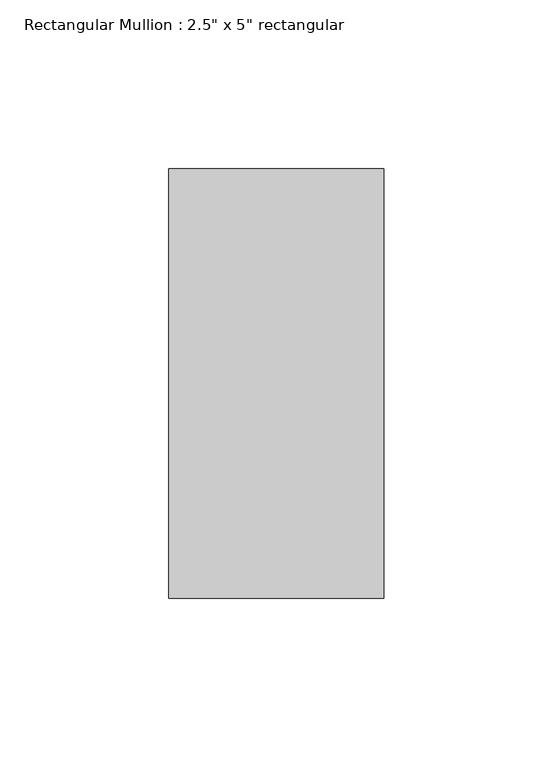
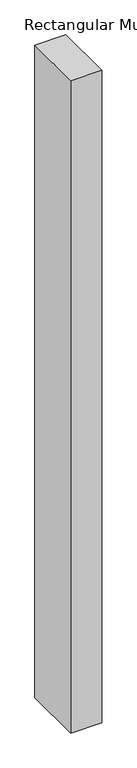
"""IFC4 building model written with IfcOpenShell, lengths in millimetres: member geometry."""

from ifc_helpers import new_model, si_unit, frame, origin, place, context, project, spatial, polyline, outline, extrude, source, transform, mapped, element, save


def member_0052055d(model_context):
    return source(origin(), model_context, "Body", "SweptSolid", [
        extrude(outline(polyline([(0.0, 63.5), (0.0, -63.5), (-63.5, -63.5), (-63.5, 63.5), (0.0, 63.5)])), frame((0.0, 0.0, -1413.2420522), z_axis=(0.0, 0.0, 1.0), x_axis=(1.0, 0.0, 0.0)), (0.0, 0.0, 1.0), 1413.2420522),
    ])


if __name__ == "__main__":
    model = new_model("IFC4")
    model_context = context("Model", 3, world=origin())
    ifc_project = project(units=[si_unit("LENGTHUNIT", "METRE", prefix="MILLI")], contexts=[model_context])
    site = spatial("IfcSite", under=ifc_project)
    building = spatial("IfcBuilding", under=site)
    placement = place(None, origin())
    member_shape = member_0052055d(model_context)
    element("IfcMember", 1, ObjectType="Rectangular Mullion : 2.5\" x 5\" rectangular", at=placement, inside=building, context=model_context, shape_type="MappedRepresentation", body=[
        mapped(member_shape, transform((0.0, 0.0, 0.0), x_axis=(1.0, 0.0, 0.0), y_axis=(0.0, 1.0, 0.0), z_axis=(0.0, 0.0, 1.0))),
    ])
    save(model, "model.ifc")

# Revit data of these elements
# Type "Rectangular Mullion : 2.5\" x 5\" rectangular"
#   built-in parameter 1007304 = 0.416667 (stored number, unit not read)
#   built-in parameter 1007301 = 0.104167 (stored number, unit not read)
#   built-in parameter 1007300 = 0.104167 (stored number, unit not read)
# Element 1 (IfcMember, "Rectangular Mullion : 2.5\" x 5\" rectangular")
#   Materials on its faces: "Aluminum"
# Materials
#   "Aluminum": class "Metal", colour RGB 247 247 247, transparency 0, Description = "Aluminum 6061", Cost = 0
